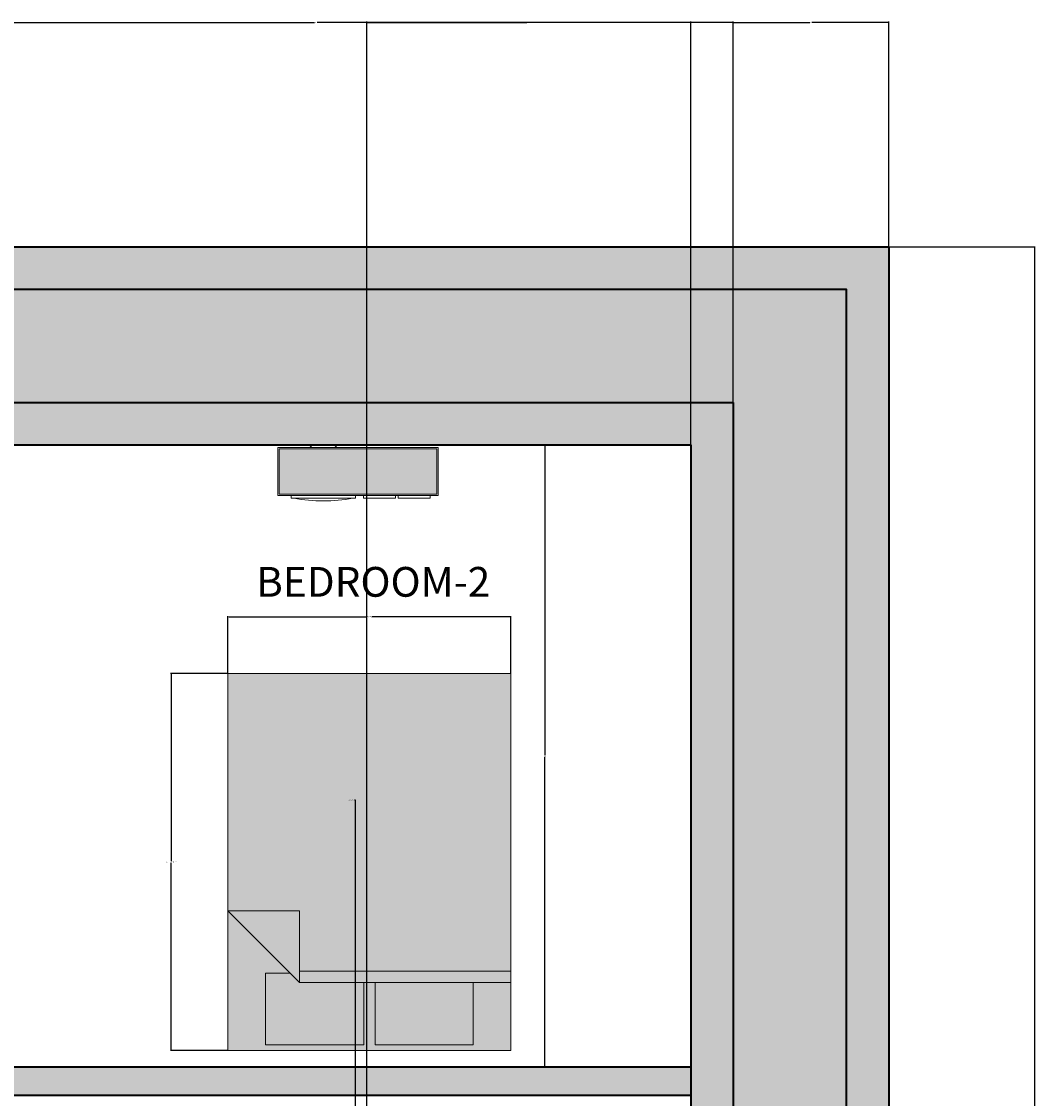
# Model space of a CAD drawing. Units: inches. Extents: x 2549 to 3108, y 1683 to 2362.
# Tile 30 of 30: x 2893 to 3108, y 2134 to 2362. Entities that reach past the tile are written whole.
import ezdxf

# ---------------------------------------------------------------- set-up
doc = ezdxf.new("R2010")
doc.units = ezdxf.units.IN
for name, color, linetype, lineweight in [('A-ANNO-DIMS', 2, 'Continuous', 18), ('A-AREA-IDEN', 7, 'Continuous', 18), ('A-FURN', 8, 'Continuous', 18), ('A-FURN-PATT', 9, 'Continuous', 13), ('A-WALL', 7, 'Continuous', 35), ('A-WALL-PATT', 89, 'Continuous', 13), ('C-PROP', 7, 'Continuous', 35)]:
    doc.layers.add(name, color=color, linetype=linetype, lineweight=lineweight)
for name, color, linetype, lineweight, true_color in [('C-PKNG-VEHI-PATT', 251, 'Continuous', 13, 0x636466), ('C-PROP-PATT', 252, 'Continuous', 13, 0x939598), ('C-PVMT-PATT', 9, 'Continuous', 13, 0xc7c8ca)]:
    doc.layers.add(name, color=color, linetype=linetype, lineweight=lineweight, true_color=true_color)
doc.styles.get("Standard").update_dxf_attribs({"font": 'arial.ttf'})
doc.dimstyles.get("Standard").update_dxf_attribs({"dimtxt": 0.18, "dimasz": 0.18, "dimexe": 0.18, "dimexo": 0.0625, "dimgap": 0.09, "dimtad": 0, "dimtih": 1, "dimtoh": 1, "dimdec": 4, "dimzin": 0, "dimdsep": 46, "dimtxsty": 'Standard', "dimcen": 0.09, "dimadec": 0, "dimazin": 0, "dimtfac": 1, "dimtdec": 4, "dimtofl": 0, "dimtmove": 0, "dimatfit": 3, "dimfxl": 1, "dimtolj": 1, "dimtzin": 0, "dimarcsym": 0})

# ---------------------------------------------------------------- blocks, each defined once
blk = doc.blocks.new('Bed - Queen')
for p, q in [((0, -80.00003), (0, 0)), ((0, 0), (59.99999, 0)), ((59.99999, 0), (59.99999, -80.00003)), ((7.99999, -1.2), (28.79998, -1.2)), ((7.99999, -14.4), (7.99999, -1.2)), ((28.79998, -1.2), (28.79998, -14.4)), ((31.19999, -1.2), (51.99999, -1.2)), ((31.19999, -14.4), (31.19999, -1.2)), ((51.99999, -1.2), (51.99999, -16.4)), ((0, -14.4), (44.8, -14.4)), ((59.99999, -29.6), (44.8, -14.4)), ((44.8, -14.4), (44.8, -29.6)), ((44.8, -16.8), (0, -16.8)), ((51.99999, -16.4), (46.79936, -16.4)), ((44.8, -29.6), (59.99999, -29.6)), ((59.99999, -80.00003), (0, -80.00003))]:
    blk.add_line(p, q)
blk = doc.blocks.new('Entertainment Center')
for p, q in [((-4, 0), (-5, -1)), ((4, 0), (-4, 0)), ((5, -1), (4, 0)), ((-17, -19), (-17, -1)), ((-17, -1), (43, -1)), ((-16.5, -18.5), (-16.5, -1.5)), ((-16.5, -1.5), (42.5, -1.5)), ((42.5, -1.5), (42.5, -18.5)), ((43, -1), (43, -19)), ((43, -19), (-17, -19)), ((42.5, -18.5), (-16.5, -18.5)), ((-12, -20), (-12, -19)), ((12, -20), (-12, -20)), ((12, -19), (12, -20)), ((15, -20), (15, -19)), ((27, -20), (15, -20)), ((27, -19), (27, -20)), ((28, -20), (28, -19)), ((40, -20), (28, -20)), ((40, -19), (40, -20))]:
    blk.add_line(p, q)
blk.add_arc((0, 40), 61, 259.6111, 280.3889)
blk = doc.blocks.new('*D12')
at = {"layer": 'A-ANNO-DIMS', "color": 0, "lineweight": -2, "transparency": 16777216}
for p, q in [((2936.43, 2224.02), (2924.32, 2224.02)), ((2924.5, 2223.84), (2924.5, 2184.21)), ((2924.5, 2144.2), (2924.5, 2183.83)), ((2936.43, 2144.02), (2924.32, 2144.02))]:
    blk.add_line(p, q, dxfattribs=at)
at = {"layer": 'A-ANNO-DIMS', "color": 0, "transparency": 16777216}
for points in [[(2924.47, 2223.84), (2924.53, 2223.84), (2924.5, 2224.02)], [(2924.47, 2144.2), (2924.53, 2144.2), (2924.5, 2144.02)]]:
    blk.add_solid(points, dxfattribs=at)
at = {"layer": 'Defpoints', "color": 0, "transparency": 16777216}
for p in [(2936.5, 2224.02), (2924.5, 2144.02), (2936.5, 2144.02)]:
    blk.add_point(p, dxfattribs=at)
at = {"layer": 'A-ANNO-DIMS', "color": 0, "transparency": 16777216, "insert": (2924.5, 2184.02), "char_height": 0.18, "attachment_point": 5}
blk.add_mtext('\\A1;QUEEN BED 80 TYP.', dxfattribs=at)
blk = doc.blocks.new('*D13')
at = {"layer": 'A-ANNO-DIMS', "color": 0, "lineweight": -2, "transparency": 16777216}
for p, q in [((2936.5, 2224.08), (2936.5, 2236.2)), ((2936.68, 2236.02), (2965.97, 2236.02)), ((2996.32, 2236.02), (2967.03, 2236.02)), ((2996.5, 2224.08), (2996.5, 2236.2))]:
    blk.add_line(p, q, dxfattribs=at)
at = {"layer": 'A-ANNO-DIMS', "color": 0, "transparency": 16777216}
for points in [[(2936.68, 2236.05), (2936.68, 2235.99), (2936.5, 2236.02)], [(2996.32, 2236.05), (2996.32, 2235.99), (2996.5, 2236.02)]]:
    blk.add_solid(points, dxfattribs=at)
at = {"layer": 'Defpoints', "color": 0, "transparency": 16777216}
for p in [(2936.5, 2236.02), (2936.5, 2224.02), (2996.5, 2224.02)]:
    blk.add_point(p, dxfattribs=at)
at = {"layer": 'A-ANNO-DIMS', "color": 0, "transparency": 16777216, "insert": (2966.5, 2236.02), "char_height": 0.18, "attachment_point": 5}
blk.add_mtext('\\A1;60 TYP.', dxfattribs=at)
blk = doc.blocks.new('*D25')
at = {"layer": 'A-ANNO-DIMS', "color": 0, "lineweight": -2, "transparency": 16777216}
for p, q in [((3076.71, 2314.52), (3107.72, 2314.52)), ((3107.54, 2314.34), (3107.54, 2014.71)), ((3107.54, 1714.7), (3107.54, 2014.34)), ((3076.71, 1714.52), (3107.72, 1714.52))]:
    blk.add_line(p, q, dxfattribs=at)
at = {"layer": 'A-ANNO-DIMS', "color": 0, "transparency": 16777216}
for points in [[(3107.51, 2314.34), (3107.57, 2314.34), (3107.54, 2314.52)], [(3107.51, 1714.7), (3107.57, 1714.7), (3107.54, 1714.52)]]:
    blk.add_solid(points, dxfattribs=at)
at = {"layer": 'Defpoints', "color": 0, "transparency": 16777216}
for p in [(3076.64, 2314.52), (3107.54, 2314.52), (3076.64, 1714.52)]:
    blk.add_point(p, dxfattribs=at)
at = {"layer": 'A-ANNO-DIMS', "color": 0, "transparency": 16777216, "insert": (3107.54, 2014.52), "char_height": 0.18, "attachment_point": 5}
blk.add_mtext('\\A1;600', dxfattribs=at)
blk = doc.blocks.new('*D29')
at = {"layer": 'A-ANNO-DIMS', "color": 0, "lineweight": -2, "transparency": 16777216}
for p, q in [((2866.64, 2272.59), (2866.64, 2362.32)), ((2866.82, 2362.14), (2954.86, 2362.14)), ((3043.46, 2362.14), (2955.42, 2362.14)), ((3043.64, 2281.59), (3043.64, 2362.32))]:
    blk.add_line(p, q, dxfattribs=at)
at = {"layer": 'A-ANNO-DIMS', "color": 0, "transparency": 16777216}
for points in [[(2866.82, 2362.17), (2866.82, 2362.11), (2866.64, 2362.14)], [(3043.46, 2362.17), (3043.46, 2362.11), (3043.64, 2362.14)]]:
    blk.add_solid(points, dxfattribs=at)
at = {"layer": 'Defpoints', "color": 0, "transparency": 16777216}
for p in [(3043.64, 2362.14), (3043.64, 2281.52), (2866.64, 2272.52)]:
    blk.add_point(p, dxfattribs=at)
at = {"layer": 'A-ANNO-DIMS', "color": 0, "transparency": 16777216, "insert": (2955.14, 2362.14), "char_height": 0.18, "attachment_point": 5}
blk.add_mtext('\\A1;177', dxfattribs=at)
blk = doc.blocks.new('*D30')
at = {"layer": 'A-ANNO-DIMS', "color": 0, "lineweight": -2, "transparency": 16777216}
for p, q in [((3043.64, 2281.59), (3043.64, 2362.32)), ((3043.82, 2362.14), (3059.92, 2362.14)), ((3076.46, 2362.14), (3060.36, 2362.14)), ((3076.64, 2314.59), (3076.64, 2362.32))]:
    blk.add_line(p, q, dxfattribs=at)
at = {"layer": 'A-ANNO-DIMS', "color": 0, "transparency": 16777216}
for points in [[(3043.82, 2362.17), (3043.82, 2362.11), (3043.64, 2362.14)], [(3076.46, 2362.17), (3076.46, 2362.11), (3076.64, 2362.14)]]:
    blk.add_solid(points, dxfattribs=at)
at = {"layer": 'Defpoints', "color": 0, "transparency": 16777216}
for p in [(3076.64, 2362.14), (3076.64, 2314.52), (3043.64, 2281.52)]:
    blk.add_point(p, dxfattribs=at)
at = {"layer": 'A-ANNO-DIMS', "color": 0, "transparency": 16777216, "insert": (3060.14, 2362.14), "char_height": 0.18, "attachment_point": 5}
blk.add_mtext('\\A1;33', dxfattribs=at)
blk = doc.blocks.new('*D41')
at = {"layer": 'A-ANNO-DIMS', "color": 0, "lineweight": -2, "transparency": 16777216}
for p, q in [((3034.58, 2272.52), (3003.56, 2272.52)), ((3003.74, 2272.34), (3003.74, 2206.71)), ((3003.74, 2140.7), (3003.74, 2206.34)), ((3034.58, 2140.52), (3003.56, 2140.52))]:
    blk.add_line(p, q, dxfattribs=at)
at = {"layer": 'A-ANNO-DIMS', "color": 0, "transparency": 16777216}
for points in [[(3003.71, 2272.34), (3003.77, 2272.34), (3003.74, 2272.52)], [(3003.71, 2140.7), (3003.77, 2140.7), (3003.74, 2140.52)]]:
    blk.add_solid(points, dxfattribs=at)
at = {"layer": 'Defpoints', "color": 0, "transparency": 16777216}
for p in [(3003.74, 2272.52), (3034.64, 2272.52), (3034.64, 2140.52)]:
    blk.add_point(p, dxfattribs=at)
at = {"layer": 'A-ANNO-DIMS', "color": 0, "transparency": 16777216, "insert": (3003.74, 2206.52), "char_height": 0.18, "attachment_point": 5}
blk.add_mtext('\\A1;132', dxfattribs=at)
blk = doc.blocks.new('*D46')
at = {"layer": 'A-ANNO-DIMS', "color": 0, "lineweight": -2, "transparency": 16777216}
for p, q in [((2812.64, 2140.46), (2812.64, 1683.44)), ((3034.64, 2134.46), (3034.64, 1683.44)), ((2812.82, 1683.62), (2923.35, 1683.62)), ((3034.46, 1683.62), (2923.93, 1683.62))]:
    blk.add_line(p, q, dxfattribs=at)
at = {"layer": 'A-ANNO-DIMS', "color": 0, "transparency": 16777216}
for points in [[(2812.82, 1683.65), (2812.82, 1683.59), (2812.64, 1683.62)], [(3034.46, 1683.65), (3034.46, 1683.59), (3034.64, 1683.62)]]:
    blk.add_solid(points, dxfattribs=at)
at = {"layer": 'Defpoints', "color": 0, "transparency": 16777216}
for p in [(2812.64, 2140.52), (3034.64, 2134.52), (3034.64, 1683.62)]:
    blk.add_point(p, dxfattribs=at)
at = {"layer": 'A-ANNO-DIMS', "color": 0, "transparency": 16777216, "insert": (2923.64, 1683.62), "char_height": 0.18, "attachment_point": 5}
blk.add_mtext('\\A1;222', dxfattribs=at)
blk = doc.blocks.new('*D57')
at = {"layer": 'A-ANNO-DIMS', "color": 0, "lineweight": -2, "transparency": 16777216}
for p, q in [((2965.94, 1936.59), (2965.94, 2362.32)), ((2966.12, 2362.14), (2999.91, 2362.14)), ((3034.46, 2362.14), (3000.67, 2362.14)), ((3034.64, 1936.59), (3034.64, 2362.32))]:
    blk.add_line(p, q, dxfattribs=at)
at = {"layer": 'A-ANNO-DIMS', "color": 0, "transparency": 16777216}
for points in [[(2966.12, 2362.17), (2966.12, 2362.11), (2965.94, 2362.14)], [(3034.46, 2362.17), (3034.46, 2362.11), (3034.64, 2362.14)]]:
    blk.add_solid(points, dxfattribs=at)
at = {"layer": 'Defpoints', "color": 0, "transparency": 16777216}
for p in [(3034.64, 2362.14), (2965.94, 1936.52), (3034.64, 1936.52)]:
    blk.add_point(p, dxfattribs=at)
at = {"layer": 'A-ANNO-DIMS', "color": 0, "transparency": 16777216, "insert": (3000.29, 2362.14), "char_height": 0.18, "attachment_point": 5}
blk.add_mtext('\\A1;68.71', dxfattribs=at)
blk = doc.blocks.new('*D63')
at = {"layer": 'A-ANNO-DIMS', "color": 0, "lineweight": -2, "transparency": 16777216}
for p, q in [((2963.33, 2197.21), (2963.51, 2197.21)), ((2963.51, 2197.21), (2963.51, 2124.68)), ((2963.42, 2003.3), (2963.6, 2003.3)), ((2963.51, 2003.21), (2963.51, 2003.39))]:
    blk.add_line(p, q, dxfattribs=at)
at = {"layer": 'A-ANNO-DIMS', "color": 0, "transparency": 16777216}
blk.add_solid([(2963.54, 2124.68), (2963.48, 2124.68), (2963.51, 2124.5)], dxfattribs=at)
at = {"layer": 'Defpoints', "color": 0, "transparency": 16777216}
for p in [(2963.51, 2124.5), (2963.51, 2003.3)]:
    blk.add_point(p, dxfattribs=at)
at = {"layer": 'A-ANNO-DIMS', "color": 0, "transparency": 16777216, "insert": (2962.65, 2197.21), "char_height": 0.18, "attachment_point": 5}
blk.add_mtext('\\A1;2X R121.2', dxfattribs=at)

msp = doc.modelspace()

# ---------------------------------------------------------------- hatches: boundary and pattern name
at = {"layer": 'A-FURN-PATT', "transparency": 33554567}
h = msp.add_hatch(color=256, dxfattribs=at)
h.dxf.hatch_style = 1
h.paths.add_polyline_path([(2708.7147, 2271.6737), (2675.2813, 2271.6737), (2675.2813, 2262.0404), (2708.7147, 2262.0404)])
h.paths.add_polyline_path([(2980.8246, 2271.6737), (2947.3913, 2271.6737), (2947.3913, 2262.0404), (2980.8246, 2262.0404)])
h.paths.add_polyline_path([(2748.8496, 2101.6383), (2798.148, 2101.6383), (2798.148, 2111.4248), (2748.8496, 2111.4248)], flags=9)
h.paths.add_polyline_path([(2685.2081, 2101.489), (2719.3253, 2101.489), (2719.3253, 2111.2819), (2685.2081, 2111.2819)], flags=9)
h.paths.add_polyline_path([(2814.6852, 1907.1328), (2847.8384, 1907.1328), (2847.8384, 1916.9258), (2814.6852, 1916.9258)], flags=9)
h.paths.add_polyline_path([(2814.3906, 1835.5864), (2848.0172, 1835.5864), (2848.0172, 1845.3794), (2814.3906, 1845.3794)], flags=9)
h.paths.add_polyline_path([(2800.5245, 1759.1674), (2853.7435, 1759.1674), (2853.7435, 1768.954), (2800.5245, 1768.954)], flags=9)
h.paths.add_polyline_path([(2972.4611, 1807.3305), (3015.3943, 1807.3305), (3015.3943, 1817.117), (2972.4611, 1817.117)], flags=9)
h.paths.add_polyline_path([(2902.3327, 1888.6731), (2937.9131, 1888.6731), (2937.9131, 1898.4661), (2902.3327, 1898.4661)], flags=9)
h.paths.add_polyline_path([(2712.1779, 1878.9039), (2754.1257, 1878.9039), (2754.1257, 1888.6904), (2712.1779, 1888.6904)], flags=9)
h.paths.add_polyline_path([(2614.0056, 2012.812), (2650.0251, 2012.812), (2650.0251, 2022.4371), (2614.0056, 2022.4371)], flags=9)
h.paths.add_polyline_path([(2713.3129, 2003.1645), (2747.4237, 2003.1645), (2747.4237, 2012.951), (2713.3129, 2012.951)], flags=9)
h.paths.add_polyline_path([(2950.1379, 2001.6934), (2982.2992, 2001.6934), (2982.2992, 2011.48), (2950.1379, 2011.48)], flags=9)
h.paths.add_polyline_path([(2940.864, 2238.5537), (2997.5066, 2238.5537), (2997.5066, 2248.3466), (2940.864, 2248.3466)], flags=9)
h.paths.add_polyline_path([(2821.5457, 2202.8348), (2855.663, 2202.8348), (2855.663, 2212.6278), (2821.5457, 2212.6278)], flags=9)
h.paths.add_polyline_path([(2661.8026, 2238.6249), (2718.4451, 2238.6249), (2718.4451, 2248.4179), (2661.8026, 2248.4179)], flags=9)
h = msp.add_hatch(color=256, dxfattribs=at)
h.dxf.hatch_style = 1
h.paths.add_polyline_path([(2906.5064, 1905.2148), (2905.2584, 1904.3827), (2907.0611, 1900.7772), (2908.3092, 1901.6092)])
h.paths.add_polyline_path([(2936.522, 1914.8044), (2935.2739, 1915.6364), (2932.6391, 1912.5856), (2933.8871, 1911.7535)])
h.paths.add_polyline_path([(2950.2508, 1905.6518), (2949.0027, 1906.4839), (2947.1999, 1902.8783), (2948.448, 1902.0463)])
h.paths.add_polyline_path([(2958.5713, 1918.1326), (2956.9072, 1919.242), (2952.4696, 1908.98, 1.38742744), (2954.9657, 1907.3159)])
h.paths.add_polyline_path([(2945.2585, 1927.0078), (2943.5944, 1928.1172), (2934.9965, 1920.6287, 1.38742744), (2937.4927, 1918.9646)])
h.paths.add_polyline_path([(2748.8496, 2101.6383), (2798.148, 2101.6383), (2798.148, 2111.4248), (2748.8496, 2111.4248)], flags=9)
h.paths.add_polyline_path([(2685.2081, 2101.489), (2719.3253, 2101.489), (2719.3253, 2111.2819), (2685.2081, 2111.2819)], flags=9)
h.paths.add_polyline_path([(2814.6852, 1907.1328), (2847.8384, 1907.1328), (2847.8384, 1916.9258), (2814.6852, 1916.9258)], flags=9)
h.paths.add_polyline_path([(2814.3906, 1835.5864), (2848.0172, 1835.5864), (2848.0172, 1845.3794), (2814.3906, 1845.3794)], flags=9)
h.paths.add_polyline_path([(2800.5245, 1759.1674), (2853.7435, 1759.1674), (2853.7435, 1768.954), (2800.5245, 1768.954)], flags=9)
h.paths.add_polyline_path([(2972.4611, 1807.3305), (3015.3943, 1807.3305), (3015.3943, 1817.117), (2972.4611, 1817.117)], flags=9)
h.paths.add_polyline_path([(2902.3327, 1888.6731), (2937.9131, 1888.6731), (2937.9131, 1898.4661), (2902.3327, 1898.4661)], flags=9)
h.paths.add_polyline_path([(2712.1779, 1878.9039), (2754.1257, 1878.9039), (2754.1257, 1888.6904), (2712.1779, 1888.6904)], flags=9)
h.paths.add_polyline_path([(2614.0056, 2012.812), (2650.0251, 2012.812), (2650.0251, 2022.4371), (2614.0056, 2022.4371)], flags=9)
h.paths.add_polyline_path([(2713.3129, 2003.1645), (2747.4237, 2003.1645), (2747.4237, 2012.951), (2713.3129, 2012.951)], flags=9)
h.paths.add_polyline_path([(2950.1379, 2001.6934), (2982.2992, 2001.6934), (2982.2992, 2011.48), (2950.1379, 2011.48)], flags=9)
h.paths.add_polyline_path([(2940.864, 2238.5537), (2997.5066, 2238.5537), (2997.5066, 2248.3466), (2940.864, 2248.3466)], flags=9)
h.paths.add_polyline_path([(2821.5457, 2202.8348), (2855.663, 2202.8348), (2855.663, 2212.6278), (2821.5457, 2212.6278)], flags=9)
h.paths.add_polyline_path([(2661.8026, 2238.6249), (2718.4451, 2238.6249), (2718.4451, 2248.4179), (2661.8026, 2248.4179)], flags=9)
at = {"layer": 'A-FURN-PATT', "transparency": 33554684}
h = msp.add_hatch(color=256, dxfattribs=at)
h.dxf.hatch_style = 1
h.paths.add_polyline_path([(2722.3589, 2224.0179), (2662.3589, 2224.0179), (2662.3589, 2173.6179), (2677.5589, 2173.6179), (2677.5589, 2160.8179), (2722.3589, 2160.8179)])
h.paths.add_polyline_path([(2996.4972, 2224.0179), (2936.4972, 2224.0179), (2936.4972, 2173.6179), (2951.6972, 2173.6179), (2951.6972, 2160.8179), (2996.4972, 2160.8179)])
h = msp.add_hatch(color=256, dxfattribs=at)
h.dxf.hatch_style = 1
h.paths.add_polyline_path([(2677.5589, 2173.6179), (2662.3589, 2173.6179), (2677.5589, 2158.4179)], flags=17)
h.paths.add_polyline_path([(2662.3589, 2173.6179), (2662.3589, 2144.0179), (2722.3589, 2144.0179), (2722.3589, 2158.4179), (2714.3589, 2158.4179), (2714.3589, 2145.2179), (2693.5589, 2145.2179), (2693.5589, 2158.4179), (2691.1589, 2158.4179), (2691.1589, 2145.2179), (2670.3589, 2145.2179), (2670.3589, 2160.4179), (2675.5589, 2160.4179)])
h.paths.add_polyline_path([(2722.3589, 2160.8179), (2677.5589, 2160.8179), (2677.5589, 2158.4179), (2722.3589, 2158.4179)], flags=17)
h.paths.add_polyline_path([(2951.6972, 2173.6179), (2936.4972, 2173.6179), (2951.6972, 2158.4179)], flags=17)
h.paths.add_polyline_path([(2936.4972, 2173.6179), (2936.4972, 2144.0179), (2996.4972, 2144.0179), (2996.4972, 2158.4179), (2988.4972, 2158.4179), (2988.4972, 2145.2179), (2967.6972, 2145.2179), (2967.6972, 2158.4179), (2965.2972, 2158.4179), (2965.2972, 2145.2179), (2944.4972, 2145.2179), (2944.4972, 2160.4179), (2949.6972, 2160.4179)])
h.paths.add_polyline_path([(2996.4972, 2160.8179), (2951.6972, 2160.8179), (2951.6972, 2158.4179), (2996.4972, 2158.4179)], flags=17)
h = msp.add_hatch(color=256, dxfattribs=at)
h.dxf.hatch_style = 1
h.paths.add_polyline_path([(2691.1589, 2158.4179), (2677.5589, 2158.4179), (2675.5589, 2160.4179), (2670.3589, 2160.4179), (2670.3589, 2145.2179), (2691.1589, 2145.2179)])
h.paths.add_polyline_path([(2714.3589, 2158.4179), (2693.5589, 2158.4179), (2693.5589, 2145.2179), (2714.3589, 2145.2179)])
h.paths.add_polyline_path([(2965.2972, 2158.4179), (2951.6972, 2158.4179), (2949.6972, 2160.4179), (2944.4972, 2160.4179), (2944.4972, 2145.2179), (2965.2972, 2145.2179)])
h.paths.add_polyline_path([(2988.4972, 2158.4179), (2967.6972, 2158.4179), (2967.6972, 2145.2179), (2988.4972, 2145.2179)])
at = {"layer": 'A-WALL-PATT'}
h = msp.add_hatch(color=256, dxfattribs=at)
h.dxf.hatch_style = 1
h.paths.add_polyline_path([(2638.6427, 2272.5237), (3034.6427, 2272.5237), (3034.6427, 1936.5237), (3043.6427, 1936.5237), (3043.6427, 2281.5237), (2629.6427, 2281.5237), (2629.6427, 2074.5237), (2812.6427, 2074.5237), (2812.6427, 2140.5237), (2785.7177, 2140.5237), (2785.7177, 2134.5237), (2806.6427, 2134.5237), (2806.6427, 2080.5237), (2638.6427, 2080.5237)])
h.paths.add_polyline_path([(2638.6427, 1972.5237), (2662.6427, 1972.5237), (2662.6427, 2041.0557), (2653.6427, 2041.0557), (2653.6427, 1978.5237), (2629.6427, 1978.5237), (2629.6427, 1795.5237), (2662.6427, 1795.5237), (2881.6427, 1795.5237), (2881.6427, 1936.5237), (2965.9351, 1936.5237), (2965.9351, 1974.5439), (2959.9351, 1974.5439), (2959.9351, 1945.5237), (2881.6427, 1945.5237), (2872.6427, 1945.5237), (2872.6427, 1804.5237), (2662.6427, 1804.5237), (2638.6427, 1804.5237)])
h = msp.add_hatch(color=256, dxfattribs=at)
h.dxf.hatch_style = 1
h.paths.add_polyline_path([(2812.6427, 2272.5237), (2806.6427, 2272.5237), (2806.6427, 2182.5237), (2815.3646, 2182.5237), (2815.3646, 2188.5237), (2812.6427, 2188.5237)])
h.paths.add_polyline_path([(2872.6427, 2272.5237), (2866.6427, 2272.5237), (2866.6427, 2188.5237), (2837.9934, 2188.5237), (2837.9934, 2182.5237), (2872.6427, 2182.5237)])
h.paths.add_polyline_path([(3034.6427, 2140.5237), (2866.6427, 2140.5237), (2866.6427, 2134.5237), (3034.6427, 2134.5237)])
at = {"layer": 'C-PKNG-VEHI-PATT'}
h = msp.add_hatch(color=256, dxfattribs=at)
h.dxf.hatch_style = 1
edge = h.paths.add_edge_path()
edge.add_ellipse((2935.7258, 1791.964), major_axis=(-50.66, 0), ratio=0.84230387, start_angle=248.165046, end_angle=265.722579)
edge.add_line((2938.911, 1834.5507), (2925.8653, 1834.5507))
edge.add_ellipse((2929.0505, 1791.964), major_axis=(50.66, 0), ratio=0.84230387, start_angle=94.277421, end_angle=111.834954)
edge.add_line((2912.8508, 1832.3947), (2914.2044, 1822.2495))
edge.add_ellipse((2930.6538, 1783.1023), major_axis=(-49.3014, 0), ratio=0.84230387, start_angle=-85.12993, end_angle=-67.208085, ccw=False)
edge.add_line((2927.1247, 1824.5225), (2937.6516, 1824.5225))
edge.add_ellipse((2934.1225, 1783.1023), major_axis=(49.3014, 0), ratio=0.84230387, start_angle=67.208085, end_angle=85.12993, ccw=False)
edge.add_line((2950.5719, 1822.2495), (2951.9255, 1832.3947))
edge = h.paths.add_edge_path()
edge.add_ellipse((2903.4793, 1857.3351), major_axis=(-34.7979, 0), ratio=0.84230387, start_angle=180, end_angle=209.43857)
edge.add_ellipse((2961.297, 1857.3351), major_axis=(34.7979, 0), ratio=0.84230387, start_angle=150.56143, end_angle=180)
edge.add_line((2926.4991, 1857.3351), (2926.4991, 1843.7609))
edge.add_ellipse((2924.1251, 1844.3143), major_axis=(-0.2209, 3.9278), ratio=0.60383358, start_angle=89.002014, end_angle=253.657408, ccw=False)
edge.add_line((2921.7512, 1844.2222), (2921.7512, 1853.3975))
edge.add_line((2921.7512, 1853.3975), (2925.269, 1855.8484))
edge.add_ellipse((2925.4782, 1855.4931), major_axis=(0.4584, 0), ratio=0.84230387, start_angle=90, end_angle=134.480211, ccw=False)
edge.add_line((2925.4782, 1855.8792), (2926.4991, 1855.8792))
edge.add_line((2926.4991, 1855.8792), (2926.4991, 1857.3351))
edge.add_ellipse((2961.297, 1857.3351), major_axis=(34.7979, 0), ratio=0.84230387, start_angle=150.56143, end_angle=180, ccw=False)
edge.add_line((2932.3882, 1873.6501), (2932.3882, 1875.7801))
edge.add_ellipse((2932.3882, 1875.3939), major_axis=(0.4584, 0), ratio=0.84230387, start_angle=90, end_angle=127.93313)
edge.add_line((2932.1366, 1875.7167), (2928.5915, 1873.7564))
edge.add_ellipse((2899.9271, 2002.4692), major_axis=(155.4756, 0), ratio=0.84230387, start_angle=-80.743434, end_angle=-77.445067, ccw=False)
edge.add_ellipse((2949.4402, 1715.2151), major_axis=(-189.1422, 0), ratio=0.84230387, start_angle=-79.790461, end_angle=-77.555373)
edge.add_ellipse((3300.3614, 1852.5642), major_axis=(-386.1662, 0), ratio=0.84230387, start_angle=-2.863715, end_angle=2.198541)
edge.add_ellipse((2929.0505, 1792.5159), major_axis=(-55.6192, 0), ratio=0.84230387, start_angle=-85.917589, end_angle=-72.280047, ccw=False)
edge.add_line((2925.7129, 1839.2798), (2939.0634, 1839.2798))
edge.add_ellipse((2935.7258, 1792.5159), major_axis=(55.6192, 0), ratio=0.84230387, start_angle=72.280047, end_angle=85.917589, ccw=False)
edge.add_ellipse((2564.4149, 1852.5642), major_axis=(-386.1662, 0), ratio=0.84230387, start_angle=177.801459, end_angle=182.863715)
edge.add_ellipse((2915.3361, 1715.2151), major_axis=(189.1422, 0), ratio=0.84230387, start_angle=77.555373, end_angle=79.790461)
edge.add_ellipse((2964.8492, 2002.4692), major_axis=(-155.4756, 0), ratio=0.84230387, start_angle=77.445067, end_angle=80.743434, ccw=False)
edge.add_line((2936.1848, 1873.7564), (2932.6397, 1875.7167))
edge.add_ellipse((2932.3882, 1875.3939), major_axis=(0.4584, 0), ratio=0.84230387, start_angle=52.06687, end_angle=90)
edge.add_line((2932.3882, 1875.7801), (2932.3882, 1873.6501))
edge.add_ellipse((2903.4793, 1857.3351), major_axis=(-34.7979, 0), ratio=0.84230387, start_angle=180, end_angle=209.43857, ccw=False)
edge.add_line((2938.2772, 1857.3351), (2938.2772, 1855.8792))
edge.add_line((2938.2772, 1855.8792), (2939.4059, 1855.8792))
edge.add_ellipse((2939.2981, 1855.4931), major_axis=(-0.4584, 0), ratio=0.84230387, start_angle=225.519789, end_angle=270, ccw=False)
edge.add_line((2939.5903, 1855.7906), (2943.0251, 1853.3975))
edge.add_line((2943.0251, 1853.3975), (2943.0251, 1844.2222))
edge.add_ellipse((2940.6512, 1844.3143), major_axis=(0.2209, 3.9278), ratio=0.60383358, start_angle=106.342592, end_angle=270.997986, ccw=False)
edge.add_line((2938.2772, 1843.7609), (2938.2772, 1857.3351))
edge = h.paths.add_edge_path()
edge.add_ellipse((2932.3882, 1865.1973), major_axis=(91.081, 0), ratio=0.84230387, start_angle=256.401865, end_angle=283.598135, ccw=False)
edge.add_line((2914.2044, 1790.0239), (2914.2044, 1778.3622))
edge.add_ellipse((2932.3882, 1853.5356), major_axis=(91.081, 0), ratio=0.84230387, start_angle=256.401865, end_angle=283.598135)
edge.add_line((2950.5719, 1778.3622), (2950.5719, 1790.0239))
edge = h.paths.add_edge_path()
edge.add_ellipse((2948.7383, 1772.3145), major_axis=(1.8336, 0), ratio=0.84230387, start_angle=0, end_angle=90)
edge.add_line((2948.7383, 1773.859), (2916.038, 1773.859))
edge.add_ellipse((2916.038, 1772.3145), major_axis=(1.8336, 0), ratio=0.84230387, start_angle=90, end_angle=180)
edge.add_line((2914.2044, 1772.3145), (2914.2044, 1760.2558))
edge.add_line((2914.2044, 1760.2558), (2950.5719, 1760.2558))
edge.add_line((2950.5719, 1760.2558), (2950.5719, 1772.3145))
h.paths.add_polyline_path([(2748.8496, 2101.6383), (2798.148, 2101.6383), (2798.148, 2111.4248), (2748.8496, 2111.4248)], flags=9)
h.paths.add_polyline_path([(2685.2081, 2101.489), (2719.3253, 2101.489), (2719.3253, 2111.2819), (2685.2081, 2111.2819)], flags=9)
h.paths.add_polyline_path([(2814.6852, 1907.1328), (2847.8384, 1907.1328), (2847.8384, 1916.9258), (2814.6852, 1916.9258)], flags=9)
h.paths.add_polyline_path([(2814.3906, 1835.5864), (2848.0172, 1835.5864), (2848.0172, 1845.3794), (2814.3906, 1845.3794)], flags=9)
h.paths.add_polyline_path([(2800.5245, 1759.1674), (2853.7435, 1759.1674), (2853.7435, 1768.954), (2800.5245, 1768.954)], flags=9)
h.paths.add_polyline_path([(2972.4611, 1807.3305), (3015.3943, 1807.3305), (3015.3943, 1817.117), (2972.4611, 1817.117)], flags=9)
h.paths.add_polyline_path([(2902.3327, 1888.6731), (2937.9131, 1888.6731), (2937.9131, 1898.4661), (2902.3327, 1898.4661)], flags=9)
h.paths.add_polyline_path([(2712.1779, 1878.9039), (2754.1257, 1878.9039), (2754.1257, 1888.6904), (2712.1779, 1888.6904)], flags=9)
h.paths.add_polyline_path([(2614.0056, 2012.812), (2650.0251, 2012.812), (2650.0251, 2022.4371), (2614.0056, 2022.4371)], flags=9)
h.paths.add_polyline_path([(2713.3129, 2003.1645), (2747.4237, 2003.1645), (2747.4237, 2012.951), (2713.3129, 2012.951)], flags=9)
h.paths.add_polyline_path([(2950.1379, 2001.6934), (2982.2992, 2001.6934), (2982.2992, 2011.48), (2950.1379, 2011.48)], flags=9)
h.paths.add_polyline_path([(2940.864, 2238.5537), (2997.5066, 2238.5537), (2997.5066, 2248.3466), (2940.864, 2248.3466)], flags=9)
h.paths.add_polyline_path([(2821.5457, 2202.8348), (2855.663, 2202.8348), (2855.663, 2212.6278), (2821.5457, 2212.6278)], flags=9)
h.paths.add_polyline_path([(2661.8026, 2238.6249), (2718.4451, 2238.6249), (2718.4451, 2248.4179), (2661.8026, 2248.4179)], flags=9)
at = {"layer": 'C-PROP-PATT'}
h = msp.add_hatch(color=256, dxfattribs=at)
h.dxf.hatch_style = 1
h.paths.add_polyline_path([(3076.6427, 2314.5237), (2596.6427, 2314.5237), (2596.6427, 1714.5237), (2881.84, 1714.5237), (2881.84, 1723.5237), (2605.6427, 1723.5237), (2605.6427, 2305.5237), (3067.6427, 2305.5237), (3067.6427, 1723.5237), (3067.6427, 1714.5237), (3076.6427, 1714.5237)])
at = {"layer": 'C-PVMT-PATT'}
h = msp.add_hatch(color=256, dxfattribs=at)
h.dxf.hatch_style = 1
h.paths.add_polyline_path([(3067.6427, 2305.5237), (2605.6427, 2305.5237), (2605.6427, 2074.5237), (2629.6427, 2074.5237), (2629.6427, 2281.5237), (3043.6427, 2281.5237), (3043.6427, 1885.5237), (3043.6427, 1872.8745), (3031.1672, 1872.8745), (3031.1672, 1862.5731), (2995.8054, 1862.5731), (2995.8054, 1872.8745), (2983.1752, 1872.8745), (2983.1752, 1885.5237), (2881.6427, 1885.5237), (2881.6427, 1795.5237), (2751.0977, 1795.5237), (2751.0977, 1761.5237), (2786.1577, 1761.5237), (2786.1577, 1723.5237), (2881.84, 1723.5237), (2881.84, 1714.5237), (3067.6427, 1714.5237), (3067.6427, 1723.5237)])
edge = h.paths.add_edge_path(flags=16)
edge.add_ellipse((2949.4402, 1710.9683), major_axis=(-194.1014, 0), ratio=0.84230387, start_angle=-77.874034, end_angle=-76.219471, ccw=False)
edge.add_ellipse((2949.4402, 1715.2151), major_axis=(-189.1422, 0), ratio=0.84230387, start_angle=-79.790461, end_angle=-77.555373, ccw=False)
edge.add_ellipse((2899.9271, 2002.4692), major_axis=(155.4756, 0), ratio=0.84230387, start_angle=-80.743434, end_angle=-77.445067)
edge.add_line((2928.5915, 1873.7564), (2932.3882, 1875.8558))
edge.add_line((2932.3882, 1875.8558), (2936.1848, 1873.7564))
edge.add_ellipse((2964.8492, 2002.4692), major_axis=(-155.4756, 0), ratio=0.84230387, start_angle=77.445067, end_angle=80.743434)
edge.add_ellipse((2915.3361, 1715.2151), major_axis=(189.1422, 0), ratio=0.84230387, start_angle=77.555373, end_angle=79.790461, ccw=False)
edge.add_ellipse((2915.3361, 1710.9683), major_axis=(-194.1014, 0), ratio=0.84230387, start_angle=256.219471, end_angle=257.874034, ccw=False)
edge.add_ellipse((2628.2871, 1850.2612), major_axis=(-327.2532, 0), ratio=0.84230387, start_angle=182.17995, end_angle=183.650428, ccw=False)
edge.add_ellipse((2955.5637, 1861.9334), major_axis=(-0.9168, 0), ratio=0.84230387, start_angle=180, end_angle=270, ccw=False)
edge.add_line((2956.4805, 1862.3857), (2956.4805, 1846.4866))
edge.add_ellipse((2955.5637, 1846.939), major_axis=(-0.9168, 0), ratio=0.84230387, start_angle=90, end_angle=180, ccw=False)
edge.add_ellipse((-3607.0606, 1835.832), major_axis=(-6562.6242, 0), ratio=0.84230387, start_angle=179.61613322, end_angle=180.09022909, ccw=False)
edge.add_ellipse((2955.5637, 1791.0926), major_axis=(0.9168, 0), ratio=0.84230387, start_angle=0, end_angle=90, ccw=False)
edge.add_line((2956.4805, 1791.545), (2956.4805, 1775.6459))
edge.add_ellipse((2955.5637, 1776.0982), major_axis=(0.9168, 0), ratio=0.84230387, start_angle=270, end_angle=360, ccw=False)
edge.add_ellipse((-3607.0606, 1835.832), major_axis=(-6562.6242, 0), ratio=0.84230387, start_angle=179.3813568, end_angle=179.47172853, ccw=False)
edge.add_ellipse((2954.5907, 1763.8768), major_axis=(-1.3752, 0), ratio=0.84230387, start_angle=179.371763, end_angle=248.464757, ccw=False)
edge.add_ellipse((-3607.519, 1835.832), major_axis=(-6564.0409, 0), ratio=0.842303863, start_angle=179.35344594, end_angle=179.37176282, ccw=False)
edge.add_ellipse((2952.6829, 1761.8002), major_axis=(3.2503, 0), ratio=0.84230387, start_angle=-90, end_angle=-0.646554, ccw=False)
edge.add_line((2952.6829, 1759.0625), (2912.0934, 1759.0625))
edge.add_ellipse((2912.0934, 1761.8002), major_axis=(3.2503, 0), ratio=0.84230387, start_angle=180.646554, end_angle=270, ccw=False)
edge.add_ellipse((9472.2953, 1835.832), major_axis=(-6564.0409, 0), ratio=0.842303871, start_angle=0.62823722, end_angle=0.6465541, ccw=False)
edge.add_ellipse((2910.1856, 1763.8768), major_axis=(1.3752, 0), ratio=0.84230387, start_angle=111.535244, end_angle=180.628237, ccw=False)
edge.add_ellipse((9471.8369, 1835.832), major_axis=(-6562.6242, 0), ratio=0.84230387, start_angle=0.52827147, end_angle=0.6465541, ccw=False)
edge.add_ellipse((2909.2126, 1776.0982), major_axis=(-0.9168, 0), ratio=0.84230387, start_angle=0, end_angle=90, ccw=False)
edge.add_line((2908.2958, 1775.6459), (2908.2958, 1791.545))
edge.add_ellipse((2909.2126, 1791.0926), major_axis=(-0.9168, 0), ratio=0.84230387, start_angle=-90, end_angle=0, ccw=False)
edge.add_ellipse((9471.8369, 1835.832), major_axis=(-6562.6242, 0), ratio=0.84230387, start_angle=-0.09022909, end_angle=0.38386678, ccw=False)
edge.add_ellipse((2909.2126, 1846.939), major_axis=(-0.9168, 0), ratio=0.84230387, start_angle=0, end_angle=90, ccw=False)
edge.add_line((2908.2958, 1846.4866), (2908.2958, 1862.3857))
edge.add_ellipse((2909.2126, 1861.9334), major_axis=(0.9168, 0), ratio=0.84230387, start_angle=90, end_angle=180, ccw=False)
edge.add_ellipse((3236.4892, 1850.2612), major_axis=(327.2532, 0), ratio=0.84230387, start_angle=176.349572, end_angle=177.82005, ccw=False)
edge = h.paths.add_edge_path(flags=0)
edge.add_ellipse((2903.4793, 1857.3351), major_axis=(-34.7979, 0), ratio=0.84230387, start_angle=180, end_angle=209.43857, ccw=False)
edge.add_line((2938.2772, 1857.3351), (2938.2772, 1855.8792))
edge.add_line((2938.2772, 1855.8792), (2939.4631, 1855.8792))
edge.add_line((2939.4631, 1855.8792), (2943.0251, 1853.3975))
edge.add_line((2943.0251, 1853.3975), (2943.0251, 1844.2222))
edge.add_ellipse((2940.6512, 1844.3143), major_axis=(0.2209, 3.9278), ratio=0.60383358, start_angle=106.342592, end_angle=270.997986, ccw=False)
edge.add_line((2938.2772, 1843.7609), (2938.2772, 1857.3351))
edge.add_ellipse((2903.4793, 1857.3351), major_axis=(-34.7979, 0), ratio=0.84230387, start_angle=180, end_angle=209.43857)
edge.add_ellipse((2961.297, 1857.3351), major_axis=(34.7979, 0), ratio=0.84230387, start_angle=150.56143, end_angle=180)
edge.add_line((2926.4991, 1857.3351), (2926.4991, 1843.7609))
edge.add_ellipse((2924.1251, 1844.3143), major_axis=(-0.2209, 3.9278), ratio=0.60383358, start_angle=89.002014, end_angle=253.657408, ccw=False)
edge.add_line((2921.7512, 1844.2222), (2921.7512, 1853.3975))
edge.add_line((2921.7512, 1853.3975), (2925.3132, 1855.8792))
edge.add_line((2925.3132, 1855.8792), (2926.4991, 1855.8792))
edge.add_line((2926.4991, 1855.8792), (2926.4991, 1857.3351))
edge.add_ellipse((2961.297, 1857.3351), major_axis=(34.7979, 0), ratio=0.84230387, start_angle=150.56143, end_angle=180, ccw=False)
edge = h.paths.add_edge_path(flags=0)
edge.add_ellipse((2929.0505, 1791.964), major_axis=(50.66, 0), ratio=0.84230387, start_angle=94.277421, end_angle=111.834954, ccw=False)
edge.add_line((2925.8653, 1834.5507), (2938.911, 1834.5507))
edge.add_ellipse((2935.7258, 1791.964), major_axis=(-50.66, 0), ratio=0.84230387, start_angle=248.165046, end_angle=265.722579, ccw=False)
edge.add_line((2951.9255, 1832.3947), (2950.5719, 1822.2495))
edge.add_ellipse((2934.1225, 1783.1023), major_axis=(49.3014, 0), ratio=0.84230387, start_angle=67.208085, end_angle=85.12993)
edge.add_line((2937.6516, 1824.5225), (2927.1247, 1824.5225))
edge.add_ellipse((2930.6538, 1783.1023), major_axis=(-49.3014, 0), ratio=0.84230387, start_angle=-85.12993, end_angle=-67.208085)
edge.add_line((2914.2044, 1822.2495), (2912.8508, 1832.3947))
edge = h.paths.add_edge_path(flags=0)
edge.add_line((2910.1338, 1829.4651), (2912.6432, 1821.2711))
edge.add_ellipse((5203.7787, 1816.4367), major_axis=(-2291.1426, 0), ratio=0.84230387, start_angle=-0.1208974, end_angle=0.3640763)
edge.add_line((2912.7012, 1801.8782), (2910.3305, 1792.5698))
edge.add_ellipse((9471.8369, 1835.832), major_axis=(-6561.7074, 0), ratio=0.84230387, start_angle=0.05559431, end_angle=0.37776419, ccw=False)
edge = h.paths.add_edge_path(flags=0)
edge.add_ellipse((-3607.0606, 1835.832), major_axis=(6561.7074, 0), ratio=0.84230387, start_angle=-0.37776419, end_angle=-0.05559431, ccw=False)
edge.add_line((2954.4458, 1792.5698), (2952.0751, 1801.8782))
edge.add_ellipse((660.9976, 1816.4367), major_axis=(2291.1426, 0), ratio=0.84230387, start_angle=-0.3640763, end_angle=0.1208974)
edge.add_line((2952.1331, 1821.2711), (2954.6425, 1829.4651))
edge = h.paths.add_edge_path(flags=0)
edge.add_ellipse((2932.3882, 1865.1973), major_axis=(91.081, 0), ratio=0.84230387, start_angle=256.401865, end_angle=283.598135)
edge.add_line((2950.5719, 1790.0239), (2950.5719, 1778.3622))
edge.add_ellipse((2932.3882, 1853.5356), major_axis=(91.081, 0), ratio=0.84230387, start_angle=256.401865, end_angle=283.598135, ccw=False)
edge.add_line((2914.2044, 1778.3622), (2914.2044, 1790.0239))
edge = h.paths.add_edge_path(flags=0)
edge.add_line((2916.038, 1773.859), (2948.7383, 1773.859))
edge.add_ellipse((2948.7383, 1772.3145), major_axis=(1.8336, 0), ratio=0.84230387, start_angle=0, end_angle=90, ccw=False)
edge.add_line((2950.5719, 1772.3145), (2950.5719, 1760.2558))
edge.add_line((2950.5719, 1760.2558), (2914.2044, 1760.2558))
edge.add_line((2914.2044, 1760.2558), (2914.2044, 1772.3145))
edge.add_ellipse((2916.038, 1772.3145), major_axis=(1.8336, 0), ratio=0.84230387, start_angle=90, end_angle=180, ccw=False)
h.paths.add_polyline_path([(2629.6427, 1978.5237), (2605.6427, 1978.5237), (2605.6427, 1723.5237), (2629.6427, 1723.5237), (2629.6427, 1795.5237)], flags=17)
h.paths.add_polyline_path([(2800.5245, 1759.1674), (2853.7435, 1759.1674), (2853.7435, 1768.954), (2800.5245, 1768.954)], flags=24)
h.paths.add_polyline_path([(2972.4611, 1807.3305), (3015.3943, 1807.3305), (3015.3943, 1817.117), (2972.4611, 1817.117)], flags=24)

# ---------------------------------------------------------------- linework, layer by layer
at = {"layer": 'A-WALL'}
for p, q in [((2629.6427, 2281.5237), (3043.6427, 2281.5237)), ((3043.6427, 2281.5237), (3043.6427, 1885.5237)), ((2638.6427, 2272.5237), (3034.6427, 2272.5237)), ((3034.6427, 2272.5237), (3034.6427, 1936.5237)), ((2866.6427, 2140.5237), (3034.6427, 2140.5237)), ((2866.6427, 2134.5237), (3034.6427, 2134.5237))]:
    msp.add_line(p, q, dxfattribs=at)
at = {"layer": 'C-PROP'}
msp.add_lwpolyline([(2596.6427, 2314.5237), (3076.6427, 2314.5237), (3076.6427, 1714.5237), (2596.6427, 1714.5237)], close=True, dxfattribs=at)
msp.add_lwpolyline([(2881.84, 1723.5237), (2605.6427, 1723.5237), (2605.6427, 2305.5237), (3067.6427, 2305.5237), (3067.6427, 1723.5237)], dxfattribs=at)

# ---------------------------------------------------------------- block references
at = {"layer": 'A-FURN', "xscale": 0.5666666666666667, "yscale": 0.5666666666666667, "zscale": 0.5666666666666667}
msp.add_blockref('Entertainment Center', (2956.7413, 2272.5237), dxfattribs=at)
at = {"layer": 'A-FURN', "rotation": 180}
msp.add_blockref('Bed - Queen', (2996.4972, 2144.0179), dxfattribs=at)

# ---------------------------------------------------------------- texts
at = {"layer": 'A-AREA-IDEN'}
msp.add_text('BEDROOM-2', height=6.30916, dxfattribs=at).set_placement((2942.4962, 2240.2934))

# ---------------------------------------------------------------- dimensions: what is measured, and where the dimension line sits
at = {"layer": 'A-ANNO-DIMS'}
for base, p1, p2, override, picture, middle in [((3043.6427, 2362.1425), (2866.6427, 2272.5237), (3043.6427, 2281.5237), {"dimdec": 0, "dimlfac": 1, "dimrnd": 0, "dimzin": 0, "dimdsep": 46, "dimlunit": 2}, '*D29', (2955.1427, 2362.1425)), ((3034.6427, 2362.1425), (2965.9351, 1936.5237), (3034.6427, 1936.5237), {"dimdec": 2, "dimlfac": 1, "dimrnd": 0, "dimzin": 0, "dimdsep": 46, "dimlunit": 2}, '*D57', (3000.2889, 2362.1425)), ((3076.6427, 2362.1425), (3043.6427, 2281.5237), (3076.6427, 2314.5237), {"dimdec": 0, "dimlfac": 1, "dimrnd": 0, "dimzin": 0, "dimdsep": 46, "dimlunit": 2}, '*D30', (3060.1427, 2362.1425)), ((3034.6427, 1683.6237), (2812.6427, 2140.5237), (3034.6427, 2134.5237), {"dimdec": 0, "dimlfac": 1, "dimrnd": 0, "dimzin": 0, "dimdsep": 46, "dimlunit": 2}, '*D46', (2923.6427, 1683.6237))]:
    dim = msp.add_linear_dim(base=base, p1=p1, p2=p2, dimstyle='Standard', override=override, dxfattribs=at)
    dim.commit()
    dim.dimension.update_dxf_attribs({"geometry": picture, "text_midpoint": middle})
for base, p1, p2, picture, middle in [((3107.5427, 2314.5237), (3076.6427, 1714.5237), (3076.6427, 2314.5237), '*D25', (3107.5427, 2014.5237)), ((3003.7427, 2272.5237), (3034.6427, 2140.5237), (3034.6427, 2272.5237), '*D41', (3003.7427, 2206.5237))]:
    dim = msp.add_linear_dim(base=base, p1=p1, p2=p2, angle=90, dimstyle='Standard', override={"dimdec": 0, "dimlfac": 1, "dimrnd": 0, "dimzin": 0, "dimdsep": 46, "dimlunit": 2}, dxfattribs=at)
    dim.commit()
    dim.dimension.update_dxf_attribs({"geometry": picture, "text_midpoint": middle})
for base, p1, p2, angle, text, picture, middle in [((2936.4972, 2236.0179), (2996.4972, 2224.0179), (2936.4972, 2224.0179), 180, '<> TYP.', '*D13', (2966.4972, 2236.0179)), ((2924.4972, 2144.0179), (2936.4972, 2224.0179), (2936.4972, 2144.0179), 270, 'QUEEN BED <> TYP.', '*D12', (2924.4972, 2184.0179))]:
    dim = msp.add_linear_dim(base=base, p1=p1, p2=p2, angle=angle, text=text, dimstyle='Standard', override={"dimdec": 0, "dimlfac": 1, "dimrnd": 0, "dimzin": 0, "dimdsep": 46, "dimlunit": 2}, dxfattribs=at)
    dim.commit()
    dim.dimension.update_dxf_attribs({"geometry": picture, "text_midpoint": middle})
dim = msp.add_radius_dim(center=(2963.5085, 2003.2985), mpoint=(2963.508, 2124.4953), text='2X <>', dimstyle='Standard', override={"dimdec": 1, "dimlfac": 1, "dimrnd": 0, "dimzin": 0, "dimdsep": 46, "dimlunit": 2}, dxfattribs=at)
dim.commit()
dim.dimension.update_dxf_attribs({"geometry": '*D63', "text_midpoint": (2962.6539, 2197.2134), "dimtype": 164})

doc.saveas('drawing.dxf')
